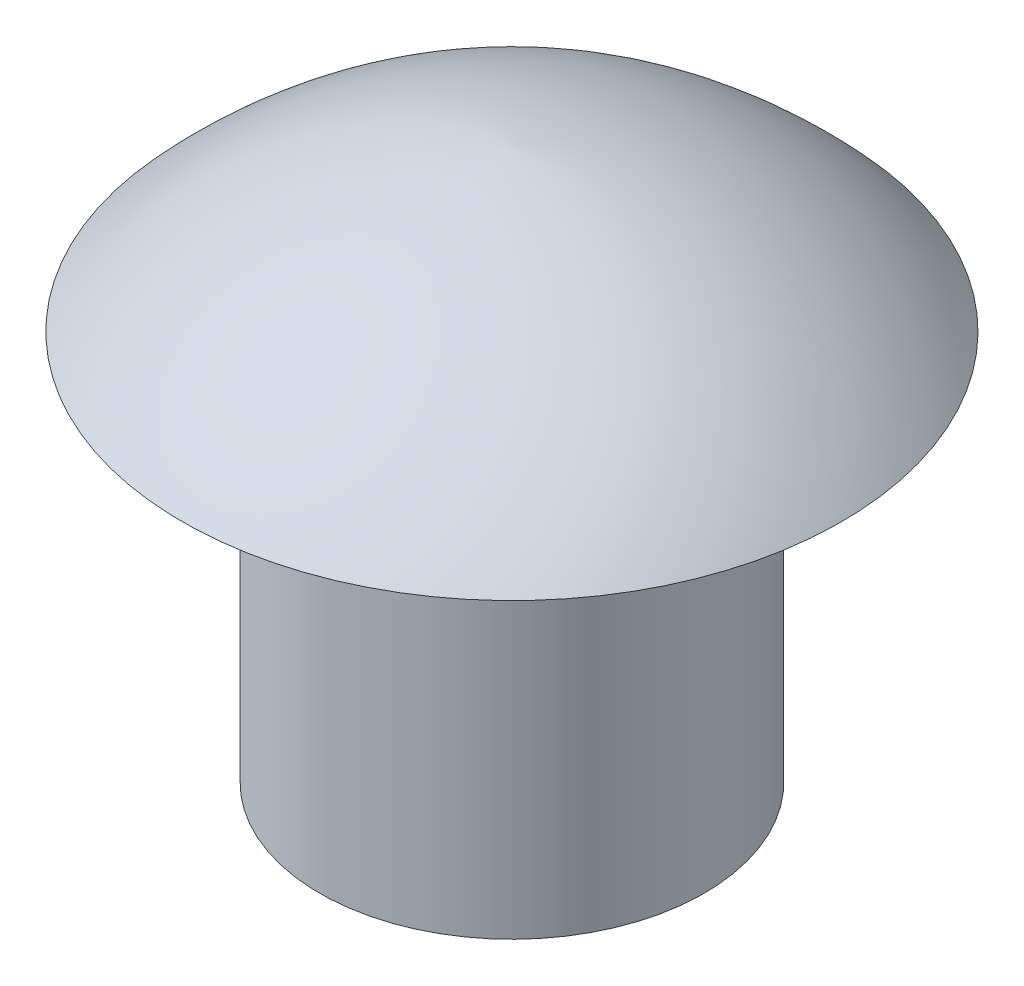
SolidWorks part; units mm, degrees
material "Plain Carbon Steel"
ref_plane "Front Plane" through (0, 0, 0) normal (0, 0, 1) x (1, 0, 0)
ref_plane "Top Plane" through (0, 0, 0) normal (0, 1, 0) x (1, 0, 0)
ref_plane "Right Plane" through (0, 0, 0) normal (1, 0, 0) x (0, 0, -1)
sketch "End Cap Half Profile" plane through (0, 0, 0) normal (0, 0, 1) x (1, 0, 0)
  line L0 (0, 0) -> (1.75, 0)
  line L1 (1.75, 0) -> (1.75, 3.5539)
  line L2 (1.75, 3.5539) -> (3, 3.5539)
  line L4 (0, 0) -> (0, 5)
  arc A0 (3, 3.5539) -> (0, 5) centre (-0.3153, 0.5111) ccw
  dimension "D3" = 4.5
  dimension "D1" = 1.75
  dimension "D2" = 3
  dimension "D4" = 5
  dimension "1.5" = 1.4461
revolve "End Cap Revolve" add sketch "End Cap Half Profile" angle 360 about L4
